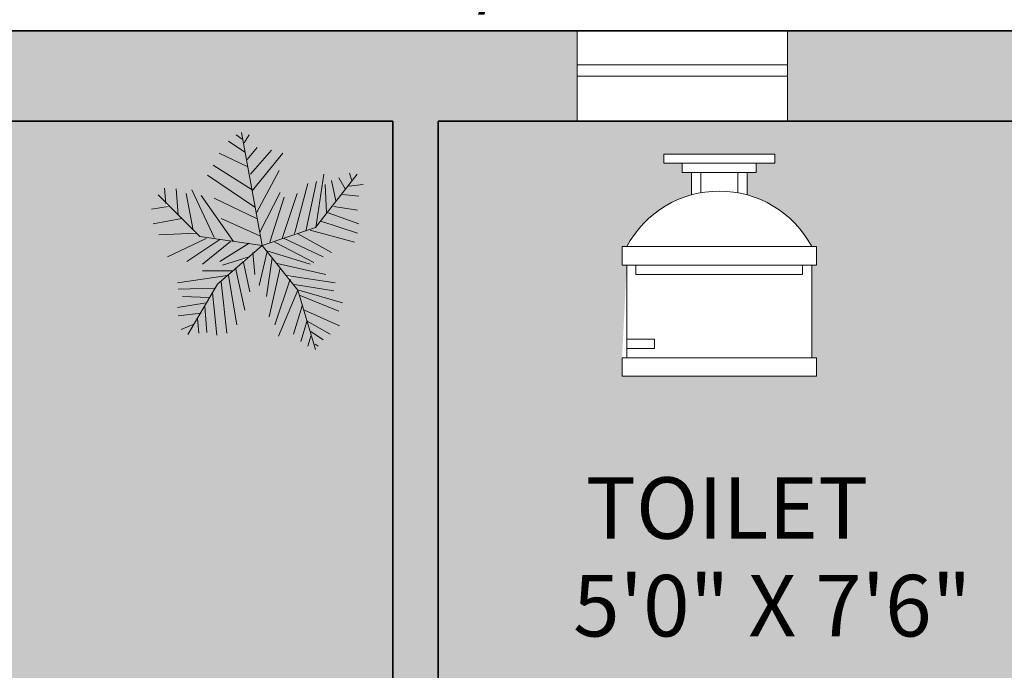
# Model space of a CAD drawing. Units: inches. Extents: x 1316 to 1777, y 813 to 1650.
# Tile 14 of 22: x 1469 to 1567, y 1512 to 1576. Entities that reach past the tile are written whole.
import ezdxf

# ---------------------------------------------------------------- set-up
doc = ezdxf.new("R2010")
doc.units = ezdxf.units.IN
doc.header["$MEASUREMENT"] = 0
for name, color, linetype, lineweight in [('A-ANNO-DIMS', 2, 'Continuous', 18), ('A-AREA-IDEN', 7, 'Continuous', 18), ('A-FLOR-FIXT', 8, 'Continuous', 18), ('A-WALL-PATT', 250, 'Continuous', 13), ('greenary', 106, 'Continuous', 13), ('walls', 250, 'Continuous', 35), ('windows', 141, 'Continuous', 18)]:
    doc.layers.add(name, color=color, linetype=linetype, lineweight=lineweight)
doc.layers.add('A-FLOR-PATT', color=254, linetype='Continuous', lineweight=13, true_color=0xfeeab9)
doc.styles.get("Standard").update_dxf_attribs({"font": 'arial.ttf'})
doc.dimstyles.get("Standard").update_dxf_attribs({"dimtxt": 7, "dimasz": 0.18, "dimexe": 0.18, "dimexo": 0.0625, "dimgap": 0.09, "dimtad": 0, "dimtih": 1, "dimtoh": 1, "dimzin": 0, "dimdsep": 46, "dimlunit": 3, "dimtxsty": 'Standard', "dimcen": 0.09, "dimadec": 0, "dimazin": 0, "dimtfac": 1, "dimtofl": 0, "dimtmove": 0, "dimatfit": 3, "dimfxl": 1, "dimtolj": 1, "dimtzin": 0, "dimarcsym": 0})

# ---------------------------------------------------------------- blocks, each defined once
blk = doc.blocks.new('*U20')
for p, q in [((-10, 22), (-10, 12)), ((10, 12), (10, 22)), ((-10, 21), (-7, 21)), ((-7, 21), (-7, 20)), ((-7, 20), (-10, 20)), ((9, 13), (-9, 13)), ((-9, 13), (-9, 12)), ((9, 12), (9, 13)), ((10.5, 12), (-10.5, 12)), ((-10.5, 10), (-10.5, 12)), ((10.5, 12), (10.5, 10)), ((10.5, 10), (-10.5, 10)), ((-3, 4.406499999999937), (-3, 2)), ((3, 2), (3, 4.406499999999937)), ((-2, 2), (-2, 4.16579999999999)), ((2, 4.16579999999999), (2, 2)), ((4, 2), (-4, 2)), ((-4, 2), (-4, 1)), ((4, 1), (4, 2))]:
    blk.add_line(p, q)
for points in [[(10.5, 22), (10.5, 24), (-10.5, 24), (-10.5, 22)], [(6, 0), (6, 1), (-6, 1), (-6, 0)]]:
    blk.add_lwpolyline(points, close=True)
blk.add_arc((0, 15.33330000000001), 11.33333, 208.0725, 331.9275)
blk = doc.blocks.new('*U13')
for p, q in [((-10.18600000000015, 53.63999999999987), (-13.08399999999983, 55.96199999999976)), ((0, 0), (-10.5, 57)), ((-9.098999999999705, 51.7819999999997), (-6.563000000000101, 55.96199999999976)), ((-8.736999999999625, 47.13799999999969), (-17.06899999999996, 52.71100000000001)), ((-7.28800000000001, 39.70699999999965), (-21.77800000000025, 46.67299999999977)), ((-7.65000000000009, 43.42299999999977), (-2.577999999999974, 49.45999999999981)), ((-5.838999999999941, 35.99199999999973), (4.666999999999916, 48.06699999999977)), ((-5.114000000000032, 27.63199999999983), (10.46300000000019, 46.67299999999977)), ((-5.114000000000032, 28.09699999999975), (-24.67599999999993, 40.63599999999996)), ((-3.665000000000418, 19.27299999999968), (-27.57400000000007, 35.52699999999982)), ((-2.940999999999803, 16.48599999999987), (8.652000000000044, 37.84999999999991)), ((27, 9), (48, 36)), ((27.12699999999995, 9.05600000000004), (31.11200000000008, 35.99199999999973)), ((44.15300000000025, 36.45599999999991), (45.23900000000003, 32.74099999999999)), ((16.25900000000001, 5.804999999999836), (23.14199999999983, 31.34799999999973)), ((22.05499999999984, 7.197999999999865), (27.48900000000003, 32.27699999999982)), ((31.83600000000024, 30.88299999999981), (32.56100000000015, 16.48599999999987)), ((35.09600000000001, 32.74099999999999), (37.26999999999998, 22.52399999999989)), ((38.71900000000005, 34.13399999999979), (41.97899999999981, 28.56099999999992)), ((43.79100000000017, 29.95399999999995), (51.03600000000006, 30.88299999999981)), ((-31.5, 4.5), (-52.5, 25.5)), ((-48.58500000000003, 21.13099999999986), (-49.30899999999974, 29.02600000000007)), ((-43.51299999999992, 28.56099999999992), (-42.42699999999968, 15.55799999999976)), ((-38.44199999999955, 26.23899999999981), (-34.81899999999996, 7.662999999999783)), ((-35.54399999999987, 28.09699999999975), (-24.31399999999985, 3.946999999999661)), ((-14.5329999999999, 2.089999999999918), (-30.83399999999983, 25.30999999999995)), ((-1.128999999999905, 6.733999999999923), (9.014000000000124, 26.70399999999995)), ((10.10100000000011, 3.482999999999719), (17.70800000000008, 26.23899999999981)), ((40.52999999999975, 25.77499999999986), (48.86200000000008, 24.846)), ((-24.31399999999985, 23.91699999999969), (-2.940999999999803, 13.69999999999982)), ((3.942000000000007, 1.625), (11.1869999999999, 24.38099999999986)), ((-47.49800000000004, 19.73699999999962), (-55.83000000000038, 18.34399999999982)), ((33.28499999999986, 16.48599999999987), (48.86200000000008, 10.91299999999978)), ((36.18300000000045, 19.73699999999962), (48.13699999999972, 17.87999999999988)), ((-40.61500000000023, 13.69999999999982), (-55.10500000000002, 10.91299999999978)), ((-20.69099999999981, 13.69999999999982), (-1.128999999999905, 4.875999999999976)), ((29.66199999999981, 12.30699999999979), (48.13699999999972, 6.268999999999778)), ((-33.37000000000035, 6.268999999999778), (-52.20699999999988, 5.339999999999918)), ((0, 0), (27, 9)), ((18.06999999999971, 5.804999999999836), (35.09600000000001, -3.483000000000174)), ((24.22899999999982, 7.662999999999783), (46.6880000000001, 1.625)), ((-28.29899999999998, 3.482999999999719), (-47.86000000000012, -5.805000000000063)), ((-21.41600000000017, 3.017999999999801), (-38.07899999999973, -8.128000000000384)), ((0, 0), (-31.5, 4.5)), ((-15.98199999999951, 2.089999999999918), (-30.11000000000013, -9.521000000000186)), ((0, 0), (-22.5, -19.5)), ((-6.563000000000101, 1.161000000000058), (-21.41600000000017, -8.128000000000384)), ((0, 0), (18, -22.5)), ((6.478000000000065, 1.625), (26.03999999999996, -8.592000000000326)), ((11.1869999999999, 3.482999999999719), (30.74900000000025, -5.805000000000063)), ((-4.751999999999952, -3.483000000000174), (-3.665000000000418, -14.62900000000013)), ((2.493000000000392, -3.019000000000005), (-1.490999999999985, -20.20200000000023)), ((1.769000000000232, -2.555000000000063), (24.22899999999982, -9.521000000000186)), ((-6.563000000000101, -5.805000000000063), (-19.96699999999964, -9.985000000000127)), ((-9.460999999999785, -8.592000000000326), (-6.201000000000021, -23.4530000000002)), ((5.028999999999996, -6.270000000000209), (2.131000000000312, -25.77500000000009)), ((7.564999999999599, -9.056000000000267), (32.19800000000032, -14.62900000000013)), ((-15.2569999999996, -12.77200000000016), (-30.11000000000013, -12.77200000000016)), ((-13.44599999999991, -11.37800000000038), (-8.736999999999625, -32.74100000000021)), ((9.014000000000124, -11.37800000000038), (3.579999999999927, -35.99200000000019)), ((-17.43100000000004, -15.09400000000005), (-42.78899999999976, -18.80899999999997)), ((-22.5, -19.5), (-37.5, -45)), ((-20.69099999999981, -18.34500000000003), (-17.79300000000012, -44.35200000000032)), ((-17.06899999999996, -15.09400000000005), (-12.721, -40.17200000000025)), ((14.08499999999958, -16.95100000000025), (6.478000000000065, -40.17200000000025)), ((12.27399999999988, -15.09400000000005), (36.9069999999997, -18.80899999999997)), ((16.25900000000001, -19.73800000000028), (36.18300000000045, -22.98900000000003)), ((-24.31399999999985, -21.59600000000023), (-42.42699999999968, -22.06000000000017)), ((-25.03800000000001, -23.91800000000035), (-22.86500000000024, -45.28100000000017)), ((18.06999999999971, -22.52400000000012), (8.289000000000215, -45.74500000000012)), ((18, -22.5), (27, -52.5)), ((18.43300000000045, -22.52400000000012), (40.52999999999975, -29.02600000000007)), ((-28.29899999999998, -29.02600000000007), (-42.78899999999976, -31.34800000000018)), ((-26.8489999999997, -26.24000000000001), (-40.25300000000015, -25.77500000000009)), ((19.1569999999997, -25.31100000000015), (38.71900000000005, -33.20600000000013)), ((-30.83399999999983, -34.13499999999999), (-42.42699999999968, -35.52800000000025)), ((-29.02300000000014, -30.88400000000002), (-27.93600000000015, -43.88700000000016)), ((20.24400000000014, -30.4190000000001), (15.89699999999993, -44.81600000000026)), ((21.33100000000013, -32.74100000000021), (39.08100000000013, -40.63600000000019)), ((-34.45699999999988, -39.70800000000031), (-40.97800000000006, -42.49400000000014)), ((-32.64600000000019, -36.92100000000005), (-31.92099999999982, -44.35200000000032)), ((22.77999999999975, -37.85000000000014), (19.51900000000023, -48.53200000000015)), ((22.77999999999975, -38.31400000000008), (34.37199999999985, -44.81600000000026)), ((24.59100000000035, -43.42300000000022), (30.74900000000025, -47.60300000000029)), ((24.59100000000035, -45.74500000000012), (23.14199999999983, -50.85400000000004)), ((26.76400000000012, -49.92500000000018), (28.21300000000019, -50.85400000000004))]:
    blk.add_line(p, q)
blk = doc.blocks.new('*D34')
at = {"layer": 'A-ANNO-DIMS', "color": 0, "lineweight": -2, "transparency": 16777216}
for p, q in [((1400.4446139869, 1575.431800926962), (1400.4446139869, 1582.375827866596)), ((1400.6246139869, 1582.195827866596), (1445.774793584458, 1582.195827866596)), ((1445.954793584458, 1575.431800926962), (1445.954793584458, 1582.375827866596)), ((1445.954793584458, 1582.195827866596), (1446.134793584458, 1582.195827866596))]:
    blk.add_line(p, q, dxfattribs=at)
at = {"layer": 'A-ANNO-DIMS', "color": 0, "transparency": 16777216}
for points in [[(1400.6246139869, 1582.225827866596), (1400.6246139869, 1582.165827866596), (1400.4446139869, 1582.195827866596)], [(1445.774793584458, 1582.225827866596), (1445.774793584458, 1582.165827866596), (1445.954793584458, 1582.195827866596)]]:
    blk.add_solid(points, dxfattribs=at)
at = {"layer": 'Defpoints', "color": 0, "transparency": 16777216}
for p in [(1445.954793584458, 1582.195827866596), (1400.4446139869, 1575.369300926962), (1445.954793584458, 1575.369300926962)]:
    blk.add_point(p, dxfattribs=at)
at = {"layer": 'A-ANNO-DIMS', "color": 0, "transparency": 16777216, "insert": (1498.669882261129, 1582.195827866596), "char_height": 7, "attachment_point": 5}
blk.add_mtext('\\A1;WINDOW 3\'-9 1/2" TYP.', dxfattribs=at)

msp = doc.modelspace()

# ---------------------------------------------------------------- hatches: boundary and pattern name
at = {"layer": 'A-FLOR-PATT'}
h = msp.add_hatch(color=256, dxfattribs=at)
h.dxf.hatch_style = 1
h.paths.add_polyline_path([(1704.173142217696, 1566.369300926962), (1574.845136951899, 1566.369300926962), (1574.845136951899, 1434.369300926962), (1704.173142217696, 1434.369300926962)])
h.paths.add_polyline_path([(1630.932461874496, 1542.855774057473), (1660.956030155827, 1542.855774057473), (1660.956030155827, 1535.715818603972), (1688.427101885747, 1535.715818603972), (1688.322102259768, 1546.60436195911), (1686.084685639232, 1547.859338051823), (1686.091126213631, 1547.880435327422), (1685.166410126033, 1550.96282228608), (1681.618706890439, 1555.397451330572), (1678.245560576594, 1552.474057858572), (1678.252731368384, 1552.432698816134), (1678.186671845043, 1552.423020957896), (1681.618706890439, 1555.397451330572), (1683.600958512701, 1556.058201871326), (1683.638878966592, 1556.171639211768), (1683.763607677471, 1556.112418259583), (1686.94026174383, 1557.171302948369), (1688.039438370375, 1558.584530039641), (1688.033686884187, 1558.6987426557), (1688.107680475544, 1558.672269889145), (1686.969155905838, 1557.208452585237), (1686.964873585789, 1557.179506895689), (1681.618706890439, 1555.397451330572), (1682.03945471648, 1554.871516548022), (1682.120272056126, 1554.846450938584), (1682.106618265419, 1554.787562111848), (1685.145085092905, 1550.989478577491), (1685.188096327656, 1550.976822603904), (1685.172977838666, 1550.940929910638), (1685.764092561596, 1548.97054750087), (1688.363951485033, 1547.81415954591), (1702.184723874646, 1547.81415954591), (1702.301389734572, 1535.715818603971), (1702.301389734572, 1481.715823291257), (1702.418055594498, 1469.617482349317), (1688.543767745673, 1469.617482349317), (1688.427101885747, 1481.715823291277), (1660.956030155827, 1481.715823291277), (1660.956030155827, 1470.852844465434), (1630.932461874496, 1470.852844465434)], flags=16)
h.paths.add_polyline_path([(1624.930620536026, 1450.279112811716), (1703.91936034353, 1450.279112810615), (1703.919360343335, 1436.319504549967), (1703.919360343529, 1435.026369171866), (1624.930620536164, 1435.026369171866), (1624.930620536164, 1435.468976146952)], flags=16)
h.paths.add_polyline_path([(1624.930620535934, 1443.713594124807), (1625.99502102627, 1443.713594124792), (1625.995021026347, 1449.228584792601), (1626.751763768497, 1449.228584792591), (1626.751763768421, 1443.713594124782), (1628.113786522866, 1443.713594124762), (1628.113786522943, 1449.228584792571), (1628.870529265094, 1449.228584792561), (1628.870529265016, 1443.713594124752), (1630.502206974044, 1443.713594124729), (1630.502206974121, 1449.228584792538), (1631.258949716271, 1449.228584792528), (1631.258949716194, 1443.713594124719), (1632.967677515695, 1443.713594124695), (1632.967677515771, 1449.228584792504), (1633.724420257922, 1449.228584792493), (1633.724420257845, 1443.713594124684), (1638.318139073099, 1443.71359412462), (1641.013180150264, 1449.599650991773), (1641.689053381981, 1449.290189808583), (1639.135704887691, 1443.713594124609), (1640.127645379921, 1443.713594124595), (1642.822686457085, 1449.599650991748), (1643.498559688802, 1449.290189808558), (1640.945211194512, 1443.713594124584), (1642.323321207278, 1443.713594124564), (1645.018362284442, 1449.599650991717), (1645.69423551616, 1449.290189808527), (1643.14088702187, 1443.713594124553), (1647.034868862889, 1443.713594124499), (1647.034868862966, 1449.228584792308), (1647.791611605116, 1449.228584792297), (1647.791611605039, 1443.713594124488), (1649.606344517206, 1443.713594124463), (1649.606344517283, 1449.228584792271), (1650.363087259433, 1449.228584792261), (1650.363087259356, 1443.713594124452), (1652.864535573064, 1443.713594124417), (1652.86453557314, 1449.228584792227), (1653.621278315291, 1449.228584792216), (1653.621278315213, 1443.713594124407), (1657.035058236599, 1443.713594124359), (1657.035058236676, 1449.228584792168), (1657.791800978826, 1449.228584792157), (1657.791800978749, 1443.713594124349), (1660.082736745753, 1443.713594124317), (1660.08273674583, 1449.228584792125), (1660.839479487981, 1449.228584792115), (1660.839479487904, 1443.713594124306), (1662.604942004505, 1443.713594124282), (1662.604942004582, 1449.228584792091), (1663.361684746731, 1449.22858479208), (1663.361684746655, 1443.713594124271), (1667.701933018638, 1443.71359412421), (1667.701933018715, 1449.228584792019), (1668.458675760865, 1449.228584792008), (1668.458675760788, 1443.7135941242), (1671.654902823707, 1443.713594124155), (1670.316094155395, 1449.228584791983), (1671.051478417664, 1449.407105279897), (1672.433624380832, 1443.713594124144), (1679.695593448107, 1443.713594124043), (1680.179092581217, 1449.2437371972), (1680.93295954233, 1449.177826782703), (1680.455222941554, 1443.713594124032), (1683.499753022321, 1443.71359412399), (1682.225483650305, 1448.723091425686), (1682.958871530074, 1448.909643819413), (1684.28059436644, 1443.713594123979), (1688.219132172317, 1443.713594123924), (1688.219132172395, 1449.228584791734), (1688.975874914544, 1449.228584791724), (1688.975874914468, 1443.713594123914), (1690.481907378039, 1443.713594123893), (1690.481907378116, 1449.228584791702), (1691.238650120266, 1449.228584791692), (1691.238650120189, 1443.713594123882), (1692.488012124579, 1443.713594123865), (1692.488012124656, 1449.228584791674), (1693.244754866807, 1449.228584791663), (1693.24475486673, 1443.713594123854), (1695.009222235677, 1443.71359412383), (1695.009222235755, 1449.228584791639), (1695.765964977904, 1449.228584791628), (1695.765964977828, 1443.713594123819), (1701.028667612474, 1443.713594123746), (1700.875476353593, 1443.379019460314), (1695.765964977823, 1443.379019460385), (1695.765964977718, 1435.871950703975), (1695.009222235568, 1435.871950703986), (1695.009222235673, 1443.379019460396), (1693.244754866725, 1443.379019460421), (1693.24475486662, 1435.87195070401), (1692.48801212447, 1435.871950704021), (1692.488012124574, 1443.379019460431), (1691.238650120184, 1443.379019460448), (1691.238650120079, 1435.871950704039), (1690.481907377929, 1435.871950704049), (1690.481907378034, 1443.379019460459), (1688.975874914463, 1443.37901946048), (1688.975874914358, 1435.871950704071), (1688.219132172208, 1435.871950704081), (1688.219132172313, 1443.379019460491), (1684.365700360234, 1443.379019460544), (1686.251552017633, 1435.965226900976), (1685.518164137864, 1435.778674507249), (1683.584859016115, 1443.379019460555), (1680.425971155915, 1443.379019460599), (1679.769629866386, 1435.871950704198), (1679.015762905273, 1435.937861118695), (1679.666341662468, 1443.37901946061), (1677.601704230459, 1443.379019460639), (1677.601704230349, 1435.459733534966), (1676.844961488199, 1435.459733534977), (1676.844961488309, 1443.379019460649), (1672.51484509118, 1443.37901946071), (1674.202394444223, 1436.427451881403), (1673.467010181954, 1436.248931393489), (1671.736123534055, 1443.379019460721), (1668.458675760783, 1443.379019460766), (1668.458675760679, 1435.871950704355), (1667.701933018528, 1435.871950704365), (1667.701933018633, 1443.379019460777), (1663.36168474665, 1443.379019460837), (1663.361684746545, 1435.871950704427), (1662.604942004395, 1435.871950704438), (1662.6049420045, 1443.379019460848), (1660.839479487899, 1443.379019460873), (1660.839479487794, 1435.871950704461), (1660.082736745644, 1435.871950704471), (1660.082736745749, 1443.379019460883), (1657.791800978744, 1443.379019460915), (1657.79180097864, 1435.871950704504), (1657.03505823649, 1435.871950704514), (1657.035058236594, 1443.379019460926), (1653.621278315209, 1443.379019460973), (1653.621278315104, 1435.871950704563), (1652.864535572954, 1435.871950704574), (1652.864535573059, 1443.379019460984), (1650.363087259352, 1443.379019461018), (1650.363087259247, 1435.871950704607), (1649.606344517097, 1435.871950704617), (1649.606344517201, 1443.379019461029), (1647.791611605034, 1443.379019461055), (1647.79161160493, 1435.871950704643), (1647.03486886278, 1435.871950704654), (1647.034868862884, 1443.379019461065), (1642.987695762989, 1443.379019461121), (1639.390427205708, 1435.522468600366), (1638.714553973992, 1435.831929783556), (1642.170129948397, 1443.379019461133), (1640.792019935631, 1443.379019461152), (1637.194751378351, 1435.522468600396), (1636.518878146634, 1435.831929783587), (1639.974454121039, 1443.379019461164), (1638.98251362881, 1443.379019461177), (1635.38524507153, 1435.522468600422), (1634.709371839813, 1435.831929783612), (1638.164947814218, 1443.379019461189), (1633.72442025784, 1443.379019461251), (1633.724420257736, 1435.87195070484), (1632.967677515585, 1435.87195070485), (1632.96767751569, 1443.379019461261), (1631.25894971619, 1443.379019461285), (1631.258949716085, 1435.871950704874), (1630.502206973934, 1435.871950704885), (1630.502206974039, 1443.379019461296), (1628.870529265012, 1443.379019461319), (1628.870529264907, 1435.871950704907), (1628.113786522757, 1435.871950704918), (1628.113786522861, 1443.379019461329), (1626.751763768416, 1443.379019461348), (1626.751763768311, 1435.871950704937), (1625.995021026161, 1435.871950704948), (1625.995021026265, 1443.379019461359), (1624.93062053593, 1443.379019461374)], flags=0)
h.paths.add_polyline_path([(1683.8388184438, 1491.516940873591), (1691.02243240811, 1491.516940873591), (1691.070762458724, 1491.582489532902), (1691.070762458724, 1529.618213888147), (1699.230602800613, 1529.618213888147), (1699.230602800613, 1513.795458682787), (1691.070762458724, 1513.795458682787), (1691.070762458724, 1507.339696078951), (1699.230602800613, 1507.339696078951), (1699.230602800613, 1491.516940873591), (1691.02243240811, 1491.516940873591), (1683.8388184438, 1481.774011611434)], flags=0)
h.paths.add_polyline_path([(1691.014795269945, 1475.340823211309, -1), (1699.947028070227, 1475.340823211309, -1)], flags=0)
h.paths.add_polyline_path([(1690.898129410018, 1541.439159465963, -1), (1699.830362210301, 1541.439159465963, -1)], flags=0)
h.paths.add_polyline_path([(1505.845136951899, 1469.59112628206), (1505.845136951899, 1566.369300926962), (1386.064450217018, 1566.369300926962), (1386.064450217018, 1450.329145456028), (1465.696913734326, 1450.329145454916), (1465.696913734311, 1449.245294229286), (1466.177135312148, 1449.025415810232), (1465.696913734293, 1447.976596354367), (1465.696913734127, 1436.054730552491), (1465.69691373438, 1434.369300926962), (1505.845136951899, 1434.369300926962), (1505.845136951899, 1440.551160024325), (1476.948765455309, 1440.551160024325), (1476.948765455309, 1441.821674157348), (1476.976571263855, 1441.821674157348, -0.4000144639257896)])
edge = h.paths.add_edge_path(flags=16)
edge.add_spline(control_points=[(1456.972809125729, 1471.793867521006), (1457.023168566332, 1471.720656303634), (1457.137927411569, 1471.553822942034), (1456.942290846074, 1471.24192378408), (1456.670432209587, 1470.85108586496), (1456.942844502639, 1470.632431111965), (1457.080784081584, 1470.521712376681)], knot_values=[0, 0, 0, 0, 0.3521435018204935, 0.802462877712905, 1.439322186147505, 2.092600477110673, 2.092600477110673, 2.092600477110673, 2.092600477110673], degree=3, periodic=0)
edge.add_spline(control_points=[(1457.32475547428, 1471.793867521006), (1457.375114914907, 1471.720656303634), (1457.489873760197, 1471.55382294204), (1457.294237194615, 1471.24192378409), (1457.022378558147, 1470.851085864945), (1457.294790851223, 1470.632431111962), (1457.432730430185, 1470.521712376681)], knot_values=[0, 0, 0, 0, 0.3521435018524344, 0.8024628777664833, 1.439322186201083, 2.092600477201539, 2.092600477201539, 2.092600477201539, 2.092600477201539], degree=3, periodic=0)
edge = h.paths.add_edge_path(flags=16)
edge.add_line((1429.512779258274, 1471.793867521006), (1429.512779258274, 1482.65684634685))
edge.add_line((1429.512779258274, 1482.65684634685), (1402.041707528354, 1482.65684634685))
edge.add_line((1402.041707528354, 1482.65684634685), (1401.925041668428, 1470.55850540489))
edge.add_line((1401.925041668428, 1470.55850540489), (1388.050753819603, 1470.55850540489))
edge.add_line((1388.050753819603, 1470.55850540489), (1388.167419679529, 1482.656846346828))
edge.add_line((1388.167419679529, 1482.656846346828), (1388.167419679529, 1536.656841659541))
edge.add_line((1388.167419679529, 1536.656841659541), (1388.284085539456, 1548.755182601482))
edge.add_line((1388.284085539456, 1548.755182601482), (1402.158373388281, 1548.755182601482))
edge.add_line((1402.158373388281, 1548.755182601482), (1402.041707528354, 1536.656841659544))
edge.add_line((1402.041707528354, 1536.656841659544), (1429.512779258274, 1536.656841659544))
edge.add_line((1429.512779258274, 1536.656841659544), (1429.512779258274, 1543.796797113046))
edge.add_line((1429.512779258274, 1543.796797113046), (1456.931962466967, 1543.796797113046))
edge.add_spline(control_points=[(1456.931962466967, 1543.796797113046), (1456.986865443904, 1543.874076116505), (1457.107876047541, 1544.044405293154), (1456.910861506863, 1544.361471057989), (1456.638392620445, 1544.752143549724), (1456.910896769912, 1544.97082320328), (1457.048882861572, 1545.081554547293)], knot_values=[0, 0, 0, 0, 0.3739942808350491, 0.8243136566734239, 1.461172965108024, 2.114451256071192, 2.114451256071192, 2.114451256071192, 2.114451256071192], degree=3, periodic=0)
edge.add_spline(control_points=[(1457.400829210173, 1545.081554547293), (1457.262843118497, 1544.970823203282), (1456.990338969004, 1544.752143549739), (1457.262807855405, 1544.361471057978), (1457.459822396166, 1544.044405293151), (1457.338811792485, 1543.874076116505), (1457.283908815528, 1543.796797113046)], knot_values=[0, 0, 0, 0, 0.6532782910004561, 1.290137599435056, 1.740456975295068, 2.114451256156171, 2.114451256156171, 2.114451256156171, 2.114451256156171], degree=3, periodic=0)
edge.add_line((1457.283908815528, 1543.796797113046), (1459.536347539605, 1543.796797113046))
edge.add_line((1459.536347539605, 1543.796797113046), (1459.536347539605, 1471.793867521006))
edge.add_line((1459.536347539605, 1471.793867521006), (1429.512779258274, 1471.793867521006))
h.paths.add_polyline_path([(1406.629990970302, 1482.715034667006), (1399.446377005991, 1492.457963929164), (1399.398046955377, 1492.457963929164), (1391.238206613488, 1492.457963929164), (1391.238206613488, 1508.280719134523), (1399.398046955377, 1508.280719134523), (1399.398046955377, 1514.736481738359), (1391.238206613488, 1514.736481738359), (1391.238206613488, 1530.559236943719), (1399.398046955377, 1530.559236943719), (1399.398046955377, 1492.523512588475), (1399.446377005991, 1492.457963929164), (1406.629990970302, 1492.457963929164)], flags=0)
h.paths.add_polyline_path([(1399.454014144157, 1476.281846266881, -1), (1390.521781343874, 1476.281846266881, -1)], flags=0)
h.paths.add_polyline_path([(1390.6384472038, 1542.380182521536, -1), (1399.570680004083, 1542.380182521536, -1)], flags=0)
h.paths.add_polyline_path([(1487.293056362471, 1548.286149051947), (1487.079502016331, 1548.251927299585), (1487.103569785383, 1547.964021870899)], flags=16)
h.paths.add_polyline_path([(1491.492982446476, 1552.843098273946), (1490.887177911646, 1552.654179820082), (1490.949131147825, 1552.371760481782)], flags=16)
h.paths.add_polyline_path([(1489.965856241701, 1554.409093477953), (1489.859237467603, 1554.560966855939), (1489.717595420028, 1554.444559309621)], flags=16)
h.paths.add_polyline_path([(1497.300520669187, 1546.483185317046), (1497.294080094788, 1546.462088041448), (1497.309433365481, 1546.453476329402)], flags=16)
h.paths.add_polyline_path([(1496.386147786754, 1549.55264326925), (1492.828101345996, 1554.000201320197), (1492.655191111377, 1554.938856879555), (1492.454253708313, 1555.029495446401), (1492.589458265089, 1555.295692330835), (1491.80635643937, 1559.546816527597), (1491.869344065012, 1559.506442238776), (1491.824003397901, 1559.45101875271), (1492.828101345996, 1554.000201320197), (1494.810352968258, 1554.660951860951), (1494.848273422149, 1554.774389201393), (1494.973002133028, 1554.715168249208), (1496.010177934814, 1555.060893516469), (1496.078408037368, 1555.314097280749), (1496.340636955742, 1555.171046523446), (1498.149656199386, 1555.774052937994), (1499.248832825931, 1557.187280029266), (1499.243081339744, 1557.301492645324), (1499.317074931101, 1557.275019878769), (1498.178550361395, 1555.811202574862), (1498.174268041345, 1555.782256885313), (1492.828101345996, 1554.000201320197), (1493.248849172036, 1553.474266537646), (1493.329666511683, 1553.449200928208), (1493.316012720976, 1553.390312101472), (1495.202682324877, 1551.031975096595), (1495.701629872663, 1550.956726846686), (1495.574163147194, 1550.5676240687), (1496.354479548461, 1549.592228567115), (1496.397490783212, 1549.579572593528)], flags=16)
h.paths.add_polyline_path([(1486.021260248876, 1555.224454602706), (1485.9580139158, 1555.548733897003), (1483.595005607934, 1557.911742204869), (1483.280309209078, 1557.859129136746), (1483.243224833943, 1558.26352297886), (1486.270024687331, 1555.236723125471)], flags=16)
h.paths.add_polyline_path([(1505.845136951899, 1469.59112628206, 0.4000144639257898), (1476.976571263855, 1441.821674157348), (1505.845136951899, 1441.821674157348)], flags=17)
h = msp.add_hatch(color=256, dxfattribs=at)
h.dxf.hatch_style = 1
h.paths.add_polyline_path([(1561.016280979732, 1510.242898591528), (1561.016280979732, 1510.274875060637), (1562.477362604382, 1510.274875060637), (1562.477362604382, 1476.87872364005), (1562.477362604382, 1471.869300926962), (1529.081211183796, 1471.869300926962), (1529.081211183796, 1476.87872364005, -0.4014527144963571)])
h.paths.add_polyline_path([(1570.345136951899, 1566.369300926962), (1510.345136951899, 1566.369300926962), (1510.345136951899, 1502.15895166366), (1526.60513386119, 1502.15895166366), (1526.60513386119, 1480.003801757213), (1510.345136951899, 1480.003801757213), (1510.345136951899, 1476.369300926962), (1529.081211183796, 1476.369300926962), (1529.081211183796, 1476.87872364005, -0.4014527144963572), (1561.016280979732, 1510.242898591528), (1561.016280979732, 1510.274875060637), (1562.477362604382, 1510.274875060637), (1562.477362604382, 1476.369300926962), (1570.345136951899, 1476.369300926962)])
h.paths.add_polyline_path([(1528.659165159676, 1540.981508023645), (1528.659165159676, 1542.824755921347), (1529.119977134102, 1552.040995409852), (1528.659165159676, 1552.040995409852), (1528.659165159676, 1553.884243307553), (1529.119964231426, 1553.884243307553, -0.2060810176159248), (1535.571344776055, 1559.041430427285), (1535.571344776055, 1561.257234898357), (1534.649720827205, 1561.257234898357), (1534.649720827205, 1562.178858847208), (1532.806472929504, 1562.178858847208), (1532.806472929504, 1563.100482796059), (1543.86596031571, 1563.100482796059), (1543.86596031571, 1562.178858847208), (1542.022712418009, 1562.178858847208), (1542.022712418009, 1561.257234898357), (1541.101088469158, 1561.257234898357), (1541.101088469158, 1559.041430427285, -0.2060810176159245), (1547.552469013788, 1553.884243307553), (1548.013268085538, 1553.884243307553), (1548.013268085538, 1552.040995409852), (1547.552456111112, 1552.040995409852), (1547.552456111112, 1542.824755921347), (1548.013268085538, 1542.824755921347), (1548.013268085538, 1540.981508023645)], flags=16)
h.paths.add_polyline_path([(1704.173142217696, 1429.869300926962), (1602.173142217695, 1429.869300926962), (1602.173142217695, 1408.281186528541), (1631.069513714286, 1408.281186528541), (1631.069513714286, 1407.010672395518), (1631.04170790574, 1407.010672395518, -0.4000144639257927), (1602.173142217695, 1379.241220270806), (1602.173142217696, 1369.869300926962), (1625.31012555338, 1369.869300926962), (1625.31012555338, 1385.783403917709), (1647.465275459828, 1385.783403917709), (1647.465275459828, 1369.869300926962), (1704.173142217696, 1369.869300926962)])
h.paths.add_polyline_path([(1669.736853868253, 1382.592842276831), (1670.236853868253, 1382.592842276831), (1670.236853868253, 1392.592842276831), (1669.736853868253, 1392.592842276831), (1669.736853868253, 1394.592842276831), (1690.736853868253, 1394.592842276831), (1690.736853868253, 1392.592842276831), (1690.236853868253, 1392.592842276831), (1690.236853868253, 1382.592842276831), (1690.736853868253, 1382.592842276831), (1690.736853868253, 1380.592842276831), (1690.236867868188, 1380.592842276831, -0.2060810176159203), (1683.236853868253, 1374.997081526295), (1683.236853868253, 1372.592842276831), (1684.236853868253, 1372.592842276831), (1684.236853868253, 1371.592842276831), (1686.236853868253, 1371.592842276831), (1686.236853868253, 1370.592842276831), (1674.236853868253, 1370.592842276831), (1674.236853868253, 1371.592842276831), (1676.236853868253, 1371.592842276831), (1676.236853868253, 1372.592842276831), (1677.236853868253, 1372.592842276831), (1677.236853868253, 1374.997081526295, -0.2060810176159203), (1670.236839868318, 1380.592842276831), (1669.736853868253, 1380.592842276831)], flags=16)
h.paths.add_polyline_path([(1631.04170790574, 1407.010672395518), (1602.029190673773, 1407.010672395518), (1602.029190673773, 1408.281186528541), (1597.673142217696, 1408.281186528541), (1597.673142217696, 1379.240863488028), (1602.029190673773, 1379.240863488028, 0.4014527144963568)])
at = {"layer": 'A-WALL-PATT'}
h = msp.add_hatch(color=256, dxfattribs=at)
h.dxf.hatch_style = 1
h.paths.add_polyline_path([(1713.173142217696, 1281.369300926962), (1656.173142217696, 1281.369300926962), (1656.173142217696, 1298.257717658217), (1651.673142217696, 1298.257717658217), (1651.673142217696, 1281.369300926962), (1567.673142217696, 1281.369300926962), (1567.673142217696, 1266.995117174766), (1572.173142217695, 1266.995117174766), (1572.173142217695, 1276.869300926963), (1704.173142217696, 1276.869300926962), (1704.173142217696, 1132.869300926962), (1608.640148269009, 1132.869300926962), (1608.640148269009, 1123.869300926962), (1704.173142217696, 1123.869300926962), (1704.173142217696, 1040.172951843256), (1652.868762127258, 1040.172951843256), (1652.868762127258, 1031.172951843254), (1713.173142217696, 1031.172951843253), (1713.173142217696, 1040.172951843256)])
h.paths.add_polyline_path([(1572.173142217696, 1237.954794134253), (1567.673142217696, 1237.954794134253), (1567.673142217696, 1123.869300926962), (1583.145592691861, 1123.869300926962), (1583.145592691861, 1132.869300926963), (1572.173142217696, 1132.869300926963)], flags=17)
h.paths.add_polyline_path([(1510.345136951899, 1566.369300926962), (1524.170902149835, 1566.369300926962), (1524.170902149835, 1571.984613741441), (1524.170902149835, 1575.369300926961), (1445.954793584458, 1575.369300926961), (1445.954793584458, 1566.369300926962), (1505.845136951899, 1566.369300926962), (1505.845136951899, 1469.591483064839), (1510.345136951899, 1469.591483064839), (1510.345136951899, 1471.869300926962), (1529.081211183796, 1471.869300926962), (1529.081211183796, 1476.369300926962), (1510.345136951899, 1476.369300926962)])
h.paths.add_polyline_path([(1609.722471703215, 1575.369300926961), (1545.118796217357, 1575.369300926961), (1545.118796217357, 1566.369300926962), (1570.345136951899, 1566.369300926962), (1570.345136951899, 1476.369300926962), (1562.477362604382, 1476.369300926962), (1562.477362604382, 1471.869300926962), (1570.345136951899, 1471.869300926962), (1570.345136951899, 1469.591483064839), (1574.845136951899, 1469.591483064839), (1574.845136951899, 1566.369300926962), (1609.722471703215, 1566.369300926962)])
h.paths.add_polyline_path([(1713.173142217696, 1575.369300926961), (1655.232651300773, 1575.369300926961), (1655.232651300773, 1566.369300926962), (1704.173142217696, 1566.369300926962), (1704.173142217696, 1434.369300926962), (1574.845136951899, 1434.369300926962), (1574.845136951899, 1440.551160024325), (1574.701185407976, 1440.551160024325), (1570.345136951899, 1440.551160024325), (1570.345136951899, 1429.869300926962), (1597.673142217696, 1429.869300926962), (1597.673142217696, 1408.281186528541), (1602.173142217695, 1408.281186528541), (1602.173142217695, 1429.869300926962), (1704.173142217696, 1429.869300926962), (1704.173142217696, 1410.703982852585), (1707.374745037781, 1410.703982852585), (1713.173142217696, 1410.703982852585)])
h.paths.add_polyline_path([(1713.173142217696, 1383.675544097327), (1704.173142217696, 1383.675544097327), (1704.173142217696, 1369.869300926962), (1602.173142217696, 1369.869300926962), (1602.173142217695, 1379.240863488028), (1597.673142217696, 1379.240863488028), (1597.673142217696, 1365.369300926962), (1713.173142217696, 1365.369300926962)])
h.paths.add_polyline_path([(1444.564450217018, 1429.869300926962), (1510.345136951899, 1429.869300926962), (1510.345136951899, 1440.551160024325), (1505.845136951899, 1440.551160024325), (1505.845136951899, 1434.369300926962), (1386.064450217018, 1434.369300926961), (1386.064450217018, 1566.369300926962), (1400.4446139869, 1566.369300926962), (1400.4446139869, 1575.369300926961), (1377.064450217018, 1575.369300926961), (1377.064450217018, 1412.813262305812), (1380.508552477466, 1412.813262305812), (1386.064450217018, 1412.813262305812), (1386.064450217018, 1429.869300926962), (1440.064450217018, 1429.869300926962), (1440.064450217018, 1401.229090636953), (1444.564450217018, 1401.229090636953)])
h.paths.add_polyline_path([(1444.564450217018, 1372.18876759644), (1440.064450217018, 1372.18876759644), (1440.064450217018, 1369.869300926962), (1386.064450217018, 1369.869300926962), (1386.064450217018, 1378.757622609401), (1377.064450217018, 1378.757622609401), (1377.064450217018, 1349.201183977028), (1381.117947355797, 1349.201183977028), (1386.064450217018, 1349.201183977028), (1386.064450217018, 1365.369300926962), (1440.064450217018, 1365.369300926962), (1440.064450217018, 1322.882360660317), (1444.564450217018, 1322.882360660317)])
h.paths.add_polyline_path([(1510.564450217018, 1295.093869264817), (1506.064450217018, 1295.093869264817), (1506.064450217018, 1245.369300926962), (1386.064450217018, 1245.369300926962), (1386.064450217018, 1272.58216425724), (1377.064450217018, 1272.58216425724), (1377.064450217018, 1212.904590025772), (1380.100240558029, 1212.904590025772), (1386.064450217018, 1212.904590025772), (1386.064450217018, 1240.869300926962), (1510.564450217018, 1240.869300926962)])
h.paths.add_polyline_path([(1386.064450217018, 1163.761289951094), (1377.064450217018, 1163.761289951094), (1377.064450217018, 1063.869300926961), (1419.36334498438, 1063.869300926961), (1419.36334498438, 1072.869300926962), (1386.064450217018, 1072.869300926962)])
h.paths.add_polyline_path([(1510.564450217018, 1072.869300926962), (1469.381492401113, 1072.869300926962), (1469.381492401113, 1063.869300926961), (1501.564450217018, 1063.869300926962), (1501.564450217018, 1033.022564166395), (1501.564450217018, 1031.172951843256), (1540.829105203347, 1031.172951843255), (1540.829105203347, 1036.182374556343, -0.0299535364659092), (1541.068383692007, 1040.172951843256), (1510.564450217018, 1040.172951843256)])
h.paths.add_polyline_path([(1607.368796217357, 1040.172951843256), (1574.225256623933, 1040.172951843256), (1574.225256623933, 1036.182374556343), (1574.225256623933, 1031.172951843255), (1607.368796217357, 1031.172951843254)], flags=17)
h.paths.add_polyline_path([(1637.054389108292, 1040.172951843256), (1624.70577568894, 1040.172951843256), (1624.70577568894, 1031.172951843254), (1637.054389108293, 1031.172951843254)], flags=17)

# ---------------------------------------------------------------- linework, layer by layer
at = {"layer": 'walls'}
for p, q in [((1377.064450217018, 1575.369300926961), (1713.173142217696, 1575.369300926961)), ((1386.064450217018, 1566.369300926962), (1505.845136951899, 1566.369300926962)), ((1505.845136951899, 1566.369300926962), (1505.845136951899, 1434.369300926962)), ((1510.345136951899, 1566.369300926962), (1510.345136951899, 1476.369300926961)), ((1510.345136951899, 1566.369300926962), (1570.345136951899, 1566.369300926962))]:
    msp.add_line(p, q, dxfattribs=at)
at = {"layer": 'windows'}
for p, q in [((1524.170902149835, 1566.369300926962), (1524.170902149835, 1575.369300926962)), ((1524.170902149835, 1575.369300926962), (1545.118796217357, 1575.369300926961)), ((1545.118796217357, 1575.369300926961), (1545.118796217357, 1566.369300926962)), ((1524.170902149835, 1566.369300926961), (1524.170902149835, 1571.984613741441)), ((1524.170902149835, 1571.984613741441), (1545.118796217357, 1571.984613741441)), ((1545.118796217357, 1571.984613741441), (1545.118796217357, 1570.869300926962)), ((1545.118796217357, 1570.869300926962), (1524.170902149835, 1570.869300926961)), ((1545.118796217357, 1566.369300926962), (1524.170902149835, 1566.369300926961))]:
    msp.add_line(p, q, dxfattribs=at)

# ---------------------------------------------------------------- block references
at = {"layer": 'A-FLOR-FIXT', "xscale": -0.9216239488505346, "yscale": 0.9216239488505346, "zscale": 0.9216239488505346, "rotation": 180}
msp.add_blockref('*U20', (1538.336216622607, 1563.100482796059), dxfattribs=at)
at = {"layer": 'greenary', "xscale": 0.1970946241996355, "yscale": 0.1970946241996355, "zscale": 0.1970946241996355}
msp.add_blockref('*U13', (1492.828101345996, 1554.000201320197), dxfattribs=at)

# ---------------------------------------------------------------- texts
at = {"layer": 'A-AREA-IDEN'}
for s, p in [('TOILET', (1525.033337454049, 1524.797944432239)), ('5\'0" X 7\'6"', (1523.780270596681, 1515.074384485459))]:
    msp.add_text(s, height=6.127076118483402, dxfattribs=at).set_placement(p)

# ---------------------------------------------------------------- dimensions: what is measured, and where the dimension line sits
at = {"layer": 'A-ANNO-DIMS'}
dim = msp.add_linear_dim(base=(1445.954793584458, 1582.195827866596), p1=(1400.4446139869, 1575.369300926962), p2=(1445.954793584458, 1575.369300926962), text='WINDOW <> TYP.', dimstyle='Standard', override={"dimdec": 1, "dimlfac": 1, "dimrnd": 0, "dimzin": 1, "dimdsep": 46, "dimlunit": 4, "dimfrac": 2}, dxfattribs=at)
dim.commit()
dim.dimension.update_dxf_attribs({"geometry": '*D34', "text_midpoint": (1498.669882261129, 1582.195827866596)})

doc.saveas('drawing.dxf')
